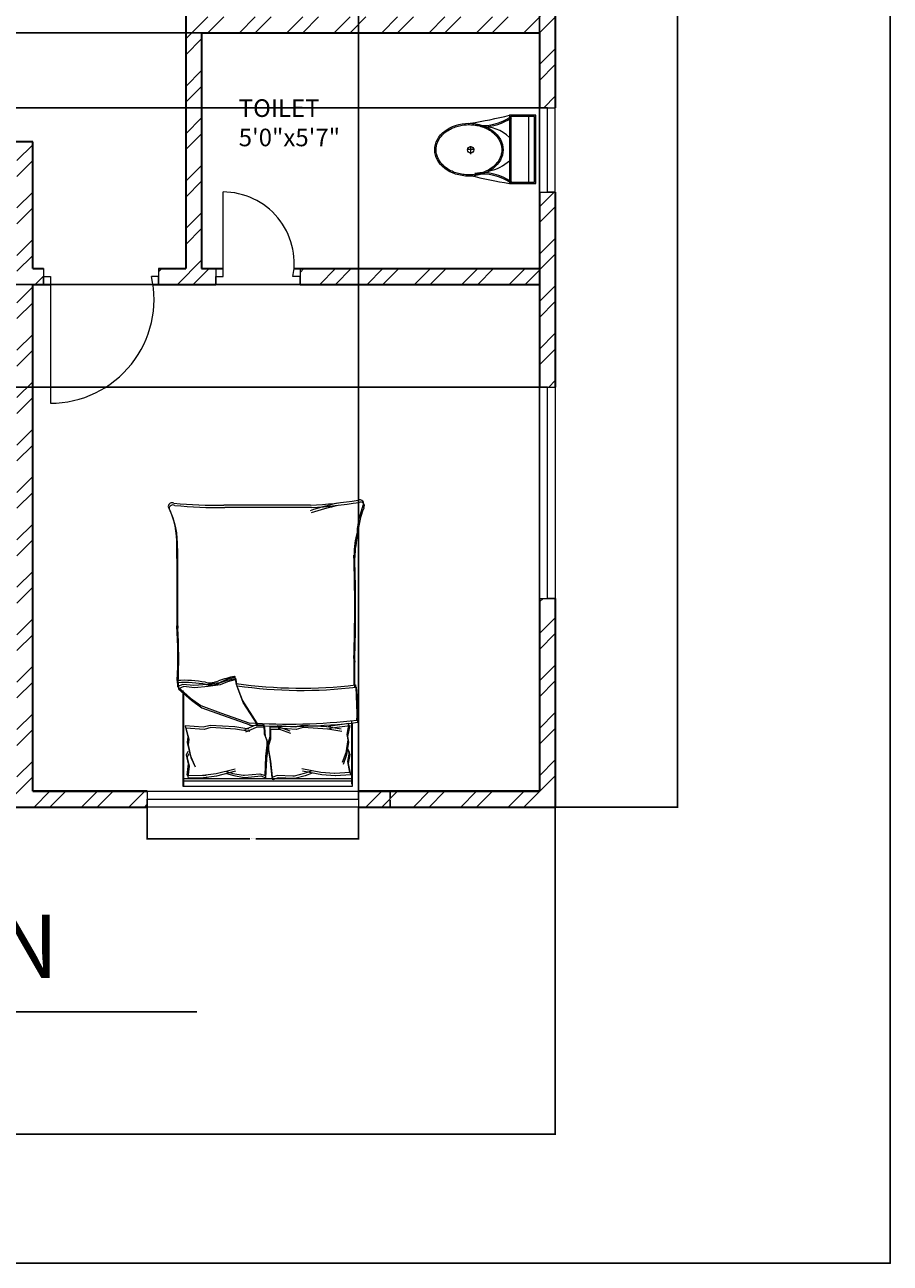
# Model space of a CAD drawing. Units: inches. Extents: x 1965 to 2673, y 1802 to 2669.
# Tile 5 of 16: x 2427 to 2673, y 1802 to 2154. Entities that reach past the tile are written whole.
import ezdxf

# ---------------------------------------------------------------- set-up
doc = ezdxf.new("R2010")
doc.units = ezdxf.units.IN
for name, color, linetype, lineweight in [('A-ANNO-DIMS', 2, 'Continuous', 18), ('A-ANNO-TTLB', 7, 'Continuous', 25), ('A-AREA-IDEN', 7, 'Continuous', 18), ('A-DOOR', 11, 'Continuous', 18), ('A-FLOR-FIXT', 9, 'Continuous', 18), ('A-FURN', 8, 'Continuous', 13), ('A-GLAZ', 181, 'Continuous', 18), ('A-WALL', 7, 'Continuous', 35), ('A-WALL-PATT', 252, 'Continuous', 13)]:
    doc.layers.add(name, color=color, linetype=linetype, lineweight=lineweight)
doc.styles.get("Standard").update_dxf_attribs({"font": 'arial.ttf'})
doc.dimstyles.get("Standard").update_dxf_attribs({"dimtxt": 0.18, "dimasz": 0.18, "dimexe": 0.18, "dimexo": 0.0625, "dimgap": 0.09, "dimtad": 0, "dimtih": 1, "dimtoh": 1, "dimdec": 4, "dimzin": 0, "dimdsep": 46, "dimtxsty": 'Standard', "dimcen": 0.09, "dimadec": 0, "dimazin": 0, "dimtfac": 1, "dimtdec": 4, "dimtofl": 0, "dimtmove": 0, "dimatfit": 3, "dimfxl": 1, "dimtolj": 1, "dimtzin": 0, "dimarcsym": 0})

# ---------------------------------------------------------------- blocks, each defined once
blk = doc.blocks.new('A$C31115884')
for p, q in [((283.1, 497.7), (223.4, 497.7)), ((257.5, 466.4), (257.5, 523.2)), ((0, 200), (0, 0)), ((520, 200), (0, 200)), ((10, 190), (10, 10)), ((510, 190), (10, 190)), ((510, 10), (510, 190)), ((520, 0), (520, 200)), ((510, 54.5), (0, 54.5)), ((10, 10), (510, 10)), ((0, 0), (520, 0))]:
    blk.add_line(p, q)
blk.add_circle((255.6, 496.4), 23.6)
for centre, radius, start, end in [((2777.7, -204.6), 2807, 165.4549, 171.71327), ((3237, 905), 2807, 188.28673, 194.5451), ((-294.5, 403.3), 364.7, 324.20913, 9.34987), ((-294.5, 403.3), 374.7, 324.20913, 9.34987), ((139.5, 406.2), 293.5, 315.84364, 2.65635), ((805.8, 403.3), 374.7, 179.20365, 215.79087), ((805.8, 403.3), 364.7, 170.65013, 215.79087), ((383.6, 406.2), 293.5, 190.27735, 224.15636)]:
    blk.add_arc(centre, radius, start, end)
blk.add_ellipse((256.2, 509.9), major_axis=(0, -260.7), ratio=0.772727)
blk.add_open_spline([(256.2, 259.2), (263.1, 259.2), (270, 259.7), (287.8, 262.3), (298.7, 265.1), (319.9, 273.1), (330.2, 278.4), (350.1, 291.1), (359.7, 298.7), (377.7, 315.9), (386.2, 325.5), (401.7, 346.6), (408.8, 358.1), (421.3, 382.5), (426.8, 395.5), (435.9, 422.4), (439.5, 436.4), (444.8, 465.1), (446.5, 479.7), (447.9, 509.2), (447.6, 524), (445, 553.3), (442.7, 567.8), (436.3, 596), (432.1, 609.7), (421.9, 636), (416, 648.6), (402.5, 672.1), (395, 683), (378.6, 703), (369.8, 712.1), (351.1, 728), (341.3, 734.8), (320.9, 746.2), (310.4, 750.7), (288.9, 757.3), (278, 759.4), (256, 761), (245, 760.6), (223.1, 757.2), (212.3, 754.3), (191.1, 746.1), (180.8, 740.7), (160.9, 727.8), (151.4, 720.1), (133.5, 702.7), (125.1, 693), (109.6, 671.7), (102.6, 660.2), (90.2, 635.7), (84.9, 622.7), (76, 595.6), (72.4, 581.6), (67.2, 552.9), (65.6, 538.2), (64.4, 508.8), (64.8, 494), (67.5, 464.7), (69.9, 450.2), (76.6, 422), (80.8, 408.3), (91.1, 382.2), (97.2, 369.7), (110.8, 346.3), (118.4, 335.4), (134.8, 315.6), (143.7, 306.7), (162.4, 290.9), (172.3, 284.2), (192.8, 273), (203.3, 268.6), (224.8, 262.2), (235.8, 260.2), (249.9, 259.3), (253, 259.2), (256.2, 259.2)], degree=3, knots=[0, 0, 0, 0, 0.110105, 0.110105, 0.285049, 0.285049, 0.459994, 0.459994, 0.634938, 0.634938, 0.809882, 0.809882, 0.984827, 0.984827, 1.159771, 1.159771, 1.334715, 1.334715, 1.50966, 1.50966, 1.684604, 1.684604, 1.859549, 1.859549, 2.034493, 2.034493, 2.209437, 2.209437, 2.384382, 2.384382, 2.559326, 2.559326, 2.73427, 2.73427, 2.909215, 2.909215, 3.084159, 3.084159, 3.259103, 3.259103, 3.434048, 3.434048, 3.608992, 3.608992, 3.783936, 3.783936, 3.958881, 3.958881, 4.133825, 4.133825, 4.30877, 4.30877, 4.483714, 4.483714, 4.658658, 4.658658, 4.833603, 4.833603, 5.008547, 5.008547, 5.183491, 5.183491, 5.358436, 5.358436, 5.53338, 5.53338, 5.708324, 5.708324, 5.883269, 5.883269, 6.058213, 6.058213, 6.233158, 6.233158, 6.283185, 6.283185, 6.283185, 6.283185])
blk = doc.blocks.new('BED-DOUBLE')
for p, q in [((3.47, 63.33), (3.47, 81.44)), ((3.47, 63.33), (3.47, 81.44)), ((3.47, 81.44), (51.49, 81.44)), ((51.26, 81.44), (51.26, 54.83)), ((51.26, 81.44), (51.26, 54.83)), ((51.49, 81.44), (51.49, 80.8)), ((3.47, 79.91), (51.26, 79.91)), ((3.47, 79.91), (51.26, 79.91)), ((3.7, 62.69), (3.7, 80.8)), ((3.7, 62.69), (3.7, 80.8)), ((3.7, 79.27), (51.49, 79.27)), ((3.7, 79.27), (51.49, 79.27)), ((3.89, 78.1), (8.17, 78.43)), ((3.89, 78.1), (8.17, 78.43)), ((3.89, 78.12), (4.47, 74.94)), ((3.89, 78.12), (4.47, 74.94)), ((4.12, 77.46), (8.4, 77.79)), ((4.12, 77.46), (8.4, 77.79)), ((4.12, 77.49), (4.7, 74.3)), ((4.12, 77.49), (4.7, 74.3)), ((8.17, 78.43), (8.28, 78.41)), ((8.17, 78.43), (8.28, 78.41)), ((8.28, 78.41), (12.1, 78.12)), ((8.28, 78.41), (12.1, 78.12)), ((8.4, 77.79), (8.51, 77.77)), ((8.4, 77.79), (8.51, 77.77)), ((8.51, 77.77), (12.33, 77.49)), ((8.51, 77.77), (12.33, 77.49)), ((12.1, 78.12), (17.6, 77.11)), ((12.1, 78.12), (17.6, 77.11)), ((12.33, 77.49), (17.82, 76.47)), ((12.33, 77.49), (17.82, 76.47)), ((14.85, 77.69), (16.87, 78.41)), ((14.85, 77.69), (16.87, 78.41)), ((15.08, 77.05), (17.1, 77.77)), ((15.08, 77.05), (17.1, 77.77)), ((16.87, 78.41), (19.76, 79.14)), ((16.87, 78.41), (19.76, 79.14)), ((17.1, 77.77), (19.99, 78.5)), ((17.1, 77.77), (19.99, 78.5)), ((19.76, 79.14), (20.09, 79.14)), ((19.76, 79.14), (20.09, 79.14)), ((19.99, 78.5), (20.31, 78.5)), ((19.99, 78.5), (20.31, 78.5)), ((20.09, 79.14), (24.53, 78.99)), ((20.09, 79.14), (24.53, 78.99)), ((20.31, 78.5), (24.76, 78.35)), ((20.31, 78.5), (24.76, 78.35)), ((24.53, 78.99), (25.98, 79.57)), ((24.53, 78.99), (25.98, 79.57)), ((24.76, 78.35), (26.21, 78.93)), ((24.76, 78.35), (26.21, 78.93)), ((25.98, 79.57), (26.56, 74.22)), ((25.98, 79.57), (26.56, 74.22)), ((26.21, 78.93), (26.78, 73.58)), ((26.21, 78.93), (26.78, 73.58)), ((27.97, 78.95), (27.73, 73.57)), ((27.97, 78.95), (27.73, 73.57)), ((28.2, 78.31), (27.96, 72.93)), ((28.2, 78.31), (27.96, 72.93)), ((29.45, 78.46), (27.97, 78.95)), ((29.45, 78.46), (27.97, 78.95)), ((29.68, 77.82), (28.2, 78.31)), ((29.68, 77.82), (28.2, 78.31)), ((33.88, 78.88), (29.45, 78.46)), ((33.88, 78.88), (29.45, 78.46)), ((34.11, 78.24), (29.68, 77.82)), ((34.11, 78.24), (29.68, 77.82)), ((34.2, 78.9), (33.88, 78.88)), ((34.2, 78.9), (33.88, 78.88)), ((34.43, 78.26), (34.11, 78.24)), ((34.43, 78.26), (34.11, 78.24)), ((37.13, 78.36), (34.2, 78.9)), ((37.13, 78.36), (34.2, 78.9)), ((37.36, 77.72), (34.43, 78.26)), ((37.36, 77.72), (34.43, 78.26)), ((41.91, 78.37), (36.49, 77.02)), ((41.91, 78.37), (36.49, 77.02)), ((42.14, 77.73), (36.72, 76.38)), ((42.14, 77.73), (36.72, 76.38)), ((39.2, 77.77), (37.13, 78.36)), ((39.19, 77.77), (37.13, 78.36)), ((39.42, 77.13), (37.36, 77.72)), ((39.42, 77.13), (37.36, 77.72)), ((45.71, 78.9), (41.91, 78.37)), ((45.71, 78.9), (41.91, 78.37)), ((45.94, 78.26), (42.14, 77.73)), ((45.94, 78.26), (42.14, 77.73)), ((50.11, 78.88), (44.7, 78.98)), ((44.7, 78.98), (45.71, 78.9)), ((50.11, 78.88), (44.7, 78.98)), ((44.7, 78.98), (45.71, 78.9)), ((50.34, 78.24), (44.93, 78.34)), ((44.93, 78.34), (45.94, 78.26)), ((50.34, 78.24), (44.93, 78.34)), ((44.93, 78.34), (45.94, 78.26)), ((50.11, 78.88), (49.73, 75.67)), ((50.11, 78.88), (49.73, 75.67)), ((50.34, 78.24), (49.96, 75.03)), ((50.34, 78.24), (49.96, 75.03)), ((51.49, 80.8), (51.49, 54.19)), ((51.49, 80.8), (51.49, 54.19)), ((4.47, 74.94), (4.03, 72.34)), ((4.47, 74.94), (4.03, 72.34)), ((4.7, 74.3), (4.26, 71.7)), ((4.7, 74.3), (4.26, 71.7)), ((5.05, 72.49), (6.06, 75.23)), ((5.05, 72.49), (6.06, 75.23)), ((5.27, 71.85), (6.29, 74.59)), ((5.27, 71.85), (6.29, 74.59)), ((26.56, 74.22), (27.13, 71.04)), ((26.56, 74.22), (27.13, 71.04)), ((49.3, 73.18), (48.12, 75.86)), ((49.3, 73.18), (48.12, 75.86)), ((49.53, 72.54), (48.35, 75.22)), ((49.53, 72.54), (48.35, 75.22)), ((49.73, 75.67), (50.32, 73.1)), ((49.73, 75.67), (50.32, 73.1)), ((49.96, 75.03), (50.55, 72.46)), ((49.96, 75.03), (50.55, 72.46)), ((4.03, 72.34), (4.61, 71.33)), ((4.03, 72.34), (4.61, 71.33)), ((4.26, 71.7), (4.84, 70.69)), ((4.26, 71.7), (4.84, 70.69)), ((4.47, 68.87), (5.05, 72.49)), ((4.47, 68.87), (5.05, 72.49)), ((4.7, 68.23), (5.27, 71.85)), ((4.7, 68.23), (5.27, 71.85)), ((26.78, 73.58), (27.36, 70.4)), ((26.78, 73.58), (27.36, 70.4)), ((27.13, 71.04), (27.13, 69.74)), ((27.13, 71.04), (27.13, 69.74)), ((27.73, 73.57), (27.35, 70.36)), ((27.73, 73.57), (27.35, 70.36)), ((27.36, 70.4), (27.36, 69.1)), ((27.36, 70.4), (27.36, 69.1)), ((27.96, 72.93), (27.58, 69.72)), ((27.96, 72.93), (27.58, 69.72)), ((50.11, 69.61), (49.3, 73.18)), ((50.11, 69.61), (49.3, 73.18)), ((50.34, 68.97), (49.53, 72.54)), ((50.34, 68.97), (49.53, 72.54)), ((50.32, 73.1), (49.81, 72.06)), ((50.32, 73.1), (49.81, 72.06)), ((50.55, 72.46), (50.04, 71.42)), ((50.55, 72.46), (50.04, 71.42)), ((4.18, 64.1), (4.76, 67.28)), ((4.18, 64.1), (4.76, 67.28)), ((4.76, 67.28), (4.47, 68.87)), ((4.76, 67.28), (4.47, 68.87)), ((4.99, 66.64), (4.7, 68.23)), ((4.99, 66.64), (4.7, 68.23)), ((27.13, 69.74), (26.56, 67.86)), ((27.13, 69.74), (26.56, 67.86)), ((26.56, 67.86), (26.56, 65.18)), ((26.56, 67.86), (26.56, 65.18)), ((27.36, 69.1), (26.78, 67.22)), ((27.36, 69.1), (26.78, 67.22)), ((26.78, 67.22), (26.78, 64.54)), ((26.78, 67.22), (26.78, 64.54)), ((27.35, 70.36), (27.43, 69.06)), ((27.35, 70.36), (27.43, 69.06)), ((27.43, 69.06), (28.13, 67.22)), ((27.43, 69.06), (28.13, 67.22)), ((27.58, 69.72), (27.66, 68.42)), ((27.58, 69.72), (27.66, 68.42)), ((27.66, 68.42), (28.35, 66.58)), ((27.66, 68.42), (28.35, 66.58)), ((28.13, 67.22), (28.29, 64.55)), ((28.13, 67.22), (28.29, 64.55)), ((49.92, 68.01), (50.11, 69.61)), ((49.92, 68.01), (50.11, 69.61)), ((50.69, 64.87), (49.92, 68.01)), ((50.69, 64.87), (49.92, 68.01)), ((50.15, 67.37), (50.34, 68.97)), ((50.15, 67.37), (50.34, 68.97)), ((50.92, 64.23), (50.15, 67.37)), ((50.92, 64.23), (50.15, 67.37)), ((9.28, 64.82), (4.18, 64.1)), ((9.28, 64.82), (4.18, 64.1)), ((4.41, 63.46), (4.99, 66.64)), ((4.41, 63.46), (4.99, 66.64)), ((9.5, 64.18), (4.41, 63.46)), ((9.5, 64.18), (4.41, 63.46)), ((6.38, 65.81), (10.41, 65.15)), ((6.38, 65.81), (10.41, 65.15)), ((6.6, 65.17), (10.64, 64.51)), ((6.61, 65.17), (10.64, 64.51)), ((10.41, 65.15), (9.28, 64.82)), ((10.41, 65.15), (9.28, 64.82)), ((10.64, 64.51), (9.5, 64.18)), ((10.64, 64.51), (9.5, 64.18)), ((10.41, 65.15), (17.42, 64.71)), ((10.41, 65.15), (17.42, 64.71)), ((10.64, 64.51), (17.65, 64.08)), ((10.64, 64.51), (17.65, 64.08)), ((17.42, 64.71), (19.38, 65.27)), ((17.42, 64.71), (19.38, 65.27)), ((17.65, 64.08), (19.61, 64.63)), ((17.65, 64.08), (19.61, 64.63)), ((19.38, 65.27), (24.51, 64.87)), ((19.38, 65.27), (24.51, 64.87)), ((19.61, 64.63), (24.74, 64.23)), ((19.61, 64.63), (24.74, 64.23)), ((24.1, 65.18), (20.95, 66.27)), ((24.1, 65.18), (20.95, 66.27)), ((24.33, 64.54), (21.18, 65.63)), ((24.33, 64.54), (21.18, 65.63)), ((26.56, 65.18), (24.1, 65.18)), ((26.56, 65.18), (24.1, 65.18)), ((26.78, 64.54), (24.33, 64.54)), ((26.78, 64.54), (24.33, 64.54)), ((28.29, 64.55), (30.75, 64.7)), ((28.29, 64.55), (30.75, 64.7)), ((28.35, 66.58), (28.52, 63.91)), ((28.35, 66.58), (28.52, 63.91)), ((28.52, 63.91), (30.97, 64.06)), ((28.52, 63.91), (30.97, 64.06)), ((30.25, 64.06), (34.44, 57.56)), ((30.25, 64.06), (34.44, 57.56)), ((30.48, 63.42), (34.67, 56.92)), ((30.48, 63.42), (34.67, 56.92)), ((30.75, 64.7), (33.82, 65.99)), ((30.75, 64.7), (33.82, 65.99)), ((30.97, 64.06), (34.04, 65.35)), ((30.97, 64.06), (34.04, 65.35)), ((40.64, 61.12), (32.3, 64.06)), ((40.64, 61.12), (32.3, 64.06)), ((40.87, 60.48), (32.53, 63.42)), ((40.87, 60.48), (32.53, 63.42)), ((32.56, 65.81), (36.59, 65.15)), ((32.56, 65.81), (36.59, 65.15)), ((32.79, 65.17), (36.82, 64.51)), ((32.79, 65.17), (36.82, 64.51)), ((36.59, 65.15), (43.6, 64.71)), ((36.59, 65.15), (43.6, 64.71)), ((36.82, 64.51), (43.83, 64.08)), ((36.82, 64.51), (43.83, 64.08)), ((43.6, 64.71), (45.56, 65.27)), ((43.6, 64.71), (45.56, 65.27)), ((43.83, 64.08), (45.79, 64.63)), ((43.83, 64.08), (45.79, 64.63)), ((45.56, 65.27), (50.69, 64.87)), ((45.56, 65.27), (50.69, 64.87)), ((45.79, 64.63), (50.92, 64.23)), ((45.79, 64.63), (50.92, 64.23)), ((46.21, 59.11), (40.64, 61.12)), ((46.21, 59.11), (40.64, 61.12)), ((46.44, 58.47), (40.87, 60.48)), ((46.44, 58.47), (40.87, 60.48)), ((34.44, 57.56), (36.15, 53.08)), ((34.44, 57.56), (36.15, 53.08)), ((34.67, 56.92), (36.38, 52.44)), ((34.67, 56.92), (36.38, 52.44)), ((49.16, 56.95), (46.21, 59.11)), ((49.16, 56.95), (46.21, 59.11)), ((49.39, 56.31), (46.44, 58.47)), ((49.39, 56.31), (46.44, 58.47)), ((52.86, 53.69), (49.16, 56.95)), ((52.86, 53.69), (49.16, 56.95)), ((53.09, 53.06), (49.39, 56.31)), ((53.09, 53.06), (49.39, 56.31)), ((36.15, 53.08), (36.46, 51.06)), ((36.15, 53.08), (36.46, 51.06)), ((40.95, 52.61), (44.36, 53.08)), ((40.95, 52.61), (44.36, 53.08)), ((44.36, 53.08), (48.23, 53.39)), ((44.36, 53.08), (48.23, 53.39)), ((48.23, 53.39), (51.33, 53.08)), ((48.23, 53.39), (51.33, 53.08)), ((51.33, 53.08), (52.86, 53.69)), ((51.33, 53.08), (52.86, 53.69)), ((51.55, 52.44), (53.09, 53.06)), ((51.55, 52.44), (53.09, 53.06)), ((52.94, 51.95), (52.86, 53.69, 3.87)), ((52.94, 51.95), (52.86, 53.69, 3.87)), ((53.17, 51.31), (53.09, 53.06, 3.87)), ((53.17, 51.31), (53.09, 53.06, 3.87)), ((36.38, 52.44), (36.69, 50.42)), ((36.38, 52.44), (36.69, 50.42)), ((36.46, 51.06), (38.94, 51.68)), ((36.46, 51.06), (38.94, 51.68)), ((36.69, 50.42), (39.16, 51.04)), ((36.69, 50.42), (39.16, 51.04)), ((38.94, 51.68), (40.95, 52.61)), ((38.94, 51.68), (40.95, 52.61)), ((39.16, 51.04), (41.18, 51.97)), ((39.16, 51.04), (41.18, 51.97)), ((41.18, 51.97), (44.58, 52.44)), ((41.18, 51.97), (44.58, 52.44)), ((44.58, 52.44), (48.46, 52.75)), ((44.58, 52.44), (48.46, 52.75)), ((48.46, 52.75), (51.55, 52.44)), ((48.46, 52.75), (51.55, 52.44)), ((15.06, 2.2), (39.67, 2.2)), ((15.06, 2.2), (39.67, 2.2)), ((15.29, 1.56), (39.9, 1.56)), ((15.29, 1.56), (39.9, 1.56))]:
    blk.add_line(p, q)
for centre, radius, start, end in [((21.35, -100.61), 164.97, 86.0865, 96.7821), ((21.35, -100.61), 164.97, 86.0865, 96.7821), ((21.58, -101.25), 164.97, 86.0865, 96.7821), ((21.58, -101.25), 164.97, 86.0865, 96.7821), ((85.16, 61.34), 83.31, 178.7218, 185.604), ((85.16, 61.34), 83.31, 178.7218, 185.604), ((85.39, 60.71), 83.31, 178.7218, 185.604), ((85.38, 60.71), 83.31, 178.7218, 185.604), ((17.75, -74.88), 129.02, 81.7845, 96.9006), ((17.75, -74.88), 129.02, 81.7845, 96.9006), ((17.98, -75.51), 129.02, 81.7845, 96.9006), ((17.98, -75.51), 129.02, 81.7845, 96.9006), ((-167.31, 50.27), 170.11, 358.4762, 1.0082), ((-167.31, 50.27), 170.11, 358.4762, 1.0082), ((-167.08, 49.63), 170.11, 358.4762, 1.0082), ((-167.08, 49.63), 170.11, 358.4762, 1.0082), ((36.63, 51), 0.185, 160.2464, 271.1377), ((36.63, 51), 0.185, 160.2464, 271.1377), ((31.15, 79.96), 29.65, 280.6617, 289.8806), ((31.15, 79.96), 29.65, 280.6617, 289.8806), ((36.86, 50.36), 0.185, 160.2464, 271.1377), ((36.86, 50.36), 0.185, 160.2464, 271.1377), ((31.38, 79.32), 29.65, 280.6617, 289.8806), ((31.38, 79.32), 29.65, 280.6617, 289.8806), ((43.74, 46.37), 6.22, 78.6608, 113.7384), ((43.74, 46.37), 6.22, 78.6608, 113.7384), ((43.97, 45.74), 6.22, 78.6608, 113.7384), ((43.97, 45.74), 6.22, 78.6608, 113.7384), ((51.32, 88.1), 36.18, 259.8763, 272.5657), ((51.32, 88.1), 36.18, 259.8763, 272.5657), ((51.55, 87.46), 36.18, 259.8763, 272.5657), ((51.55, 87.46), 36.18, 259.8763, 272.5657), ((182.26, 45.13), 129.5, 176.9791, 183.8365), ((182.26, 45.13), 129.5, 176.9791, 183.8365), ((182.49, 44.49), 129.5, 176.9791, 183.8365), ((182.49, 44.49), 129.5, 176.9791, 183.8365), ((484.82, 30.83), 482.31, 178.2277, 181.7185), ((484.82, 30.83), 482.31, 178.2277, 181.7185), ((485.05, 30.19), 482.31, 178.2277, 181.7185), ((485.05, 30.19), 482.31, 178.2277, 181.7185), ((-4508.75, 13.62), 4561.86, 0.00217, 0.28689), ((-4508.75, 13.62), 4561.86, 0.00217, 0.28689), ((-4508.52, 12.98), 4561.86, 0.00217, 0.28689), ((-4508.52, 12.98), 4561.86, 0.00217, 0.28689), ((-26.9, 16.93), 29.63, 346.0648, 358.9113), ((-26.9, 16.93), 29.63, 346.0648, 358.9113), ((-26.68, 16.29), 29.63, 346.0648, 358.9113), ((-26.68, 16.29), 29.63, 346.0648, 358.9113), ((76.15, 12.77), 23.07, 177.4714, 206.4681), ((76.15, 12.77), 23.07, 177.4714, 206.4681), ((76.38, 12.14), 23.07, 177.4714, 206.4681), ((76.38, 12.14), 23.07, 177.4714, 206.4681), ((-21.66, 11.17), 23.56, 337.9751, 356.652), ((-21.66, 11.17), 23.56, 337.9751, 356.652), ((-21.44, 10.53), 23.56, 337.9751, 356.652), ((-21.44, 10.53), 23.56, 337.9751, 356.652), ((-17.23, 105.15), 106.46, 283.3832, 287.7053), ((-17.23, 105.15), 106.46, 283.3832, 287.7053), ((1.08, 1.72), 1.09, 146.1736, 293.4781), ((1.08, 1.72), 1.09, 146.1736, 293.4781), ((1.31, 1.08), 1.09, 146.1736, 293.4781), ((1.31, 1.08), 1.09, 146.1736, 293.4781), ((21.42, -119.4), 121.76, 92.9958, 99.4091), ((21.42, -119.4), 121.76, 92.9958, 99.4091), ((21.65, -120.04), 121.76, 92.9958, 99.4091), ((21.65, -120.04), 121.76, 92.9958, 99.4091), ((-17, 104.51), 106.46, 283.3832, 287.7053), ((-17, 104.51), 106.46, 283.3832, 287.7053), ((41.15, -130.84), 133.04, 84.4998, 90.6351), ((41.15, -130.84), 133.04, 84.4998, 90.6351), ((41.38, -131.48), 133.04, 84.4998, 90.6351), ((41.37, -131.48), 133.04, 84.4998, 90.6351), ((54.4, 2.57), 1.1, 242.6588, 356.02), ((54.4, 2.57), 1.1, 242.6588, 356.02), ((54.63, 1.93), 1.1, 242.6588, 356.02), ((54.63, 1.93), 1.1, 242.6588, 356.02)]:
    blk.add_arc(centre, radius, start, end)
blk = doc.blocks.new('WIN-60IN')
for p, q in [((0, 4.5), (0, 0)), ((0, 4.5), (60, 4.5)), ((60, 2.25), (60, 4.5)), ((60, 4.5), (60, 0)), ((0, 0), (0, 2.25)), ((0, 2.25), (60, 2.25)), ((60, 0), (0, 0))]:
    blk.add_line(p, q)
blk = doc.blocks.new('WIN-24IN')
for p, q in [((0, 24), (4.5, 24)), ((0, 24), (0, 0)), ((4.5, 24), (2.25, 24)), ((2.25, 24), (2.25, 0)), ((4.5, 24), (4.5, 0)), ((2.25, 0), (0, 0)), ((0, 0), (4.5, 0))]:
    blk.add_line(p, q)
blk = doc.blocks.new('*D9')
at = {"layer": 'A-ANNO-DIMS', "color": 0, "lineweight": -2, "transparency": 16777216}
for p, q in [((2462.13, 1931.53), (2462.13, 1922.41)), ((2522.13, 1931.53), (2522.13, 1922.41)), ((2462.31, 1922.59), (2491.29, 1922.59)), ((2521.95, 1922.59), (2492.98, 1922.59))]:
    blk.add_line(p, q, dxfattribs=at)
at = {"layer": 'A-ANNO-DIMS', "color": 0, "transparency": 16777216}
for points in [[(2462.31, 1922.62), (2462.31, 1922.56), (2462.13, 1922.59)], [(2521.95, 1922.62), (2521.95, 1922.56), (2522.13, 1922.59)]]:
    blk.add_solid(points, dxfattribs=at)
at = {"layer": 'Defpoints', "color": 0, "transparency": 16777216}
for p in [(2462.13, 1931.59), (2522.13, 1931.59), (2522.13, 1922.59)]:
    blk.add_point(p, dxfattribs=at)
at = {"layer": 'A-ANNO-DIMS', "color": 0, "transparency": 16777216, "insert": (2492.13, 1922.59), "char_height": 0.18, "attachment_point": 5}
blk.add_mtext('\\A1;WIN. 60 TYP.', dxfattribs=at)
blk = doc.blocks.new('*D10')
at = {"layer": 'A-ANNO-DIMS', "color": 0, "lineweight": -2, "transparency": 16777216}
for p, q in [((2522.19, 1936.09), (2531.31, 1936.09)), ((2531.13, 1935.91), (2531.13, 1934.02)), ((2522.19, 1931.59), (2531.31, 1931.59)), ((2531.13, 1931.77), (2531.13, 1933.66))]:
    blk.add_line(p, q, dxfattribs=at)
at = {"layer": 'A-ANNO-DIMS', "color": 0, "transparency": 16777216}
for points in [[(2531.1, 1935.91), (2531.16, 1935.91), (2531.13, 1936.09)], [(2531.1, 1931.77), (2531.16, 1931.77), (2531.13, 1931.59)]]:
    blk.add_solid(points, dxfattribs=at)
at = {"layer": 'Defpoints', "color": 0, "transparency": 16777216}
for p in [(2522.13, 1936.09), (2531.13, 1936.09), (2522.13, 1931.59)]:
    blk.add_point(p, dxfattribs=at)
at = {"layer": 'A-ANNO-DIMS', "color": 0, "transparency": 16777216, "insert": (2531.13, 1933.84), "char_height": 0.18, "attachment_point": 5}
blk.add_mtext('\\A1;5 TYP.', dxfattribs=at)
blk = doc.blocks.new('*D25')
at = {"layer": 'A-ANNO-DIMS', "color": 0, "lineweight": -2, "transparency": 16777216}
for p, q in [((2047.09, 1931.53), (2047.09, 1838.49)), ((2578.09, 1931.53), (2578.09, 1838.49)), ((2047.27, 1838.67), (2312.32, 1838.67)), ((2577.91, 1838.67), (2312.86, 1838.67))]:
    blk.add_line(p, q, dxfattribs=at)
at = {"layer": 'A-ANNO-DIMS', "color": 0, "transparency": 16777216}
for points in [[(2047.27, 1838.7), (2047.27, 1838.64), (2047.09, 1838.67)], [(2577.91, 1838.7), (2577.91, 1838.64), (2578.09, 1838.67)]]:
    blk.add_solid(points, dxfattribs=at)
at = {"layer": 'Defpoints', "color": 0, "transparency": 16777216}
for p in [(2047.09, 1931.59), (2578.09, 1931.59), (2578.09, 1838.67)]:
    blk.add_point(p, dxfattribs=at)
at = {"layer": 'A-ANNO-DIMS', "color": 0, "transparency": 16777216, "insert": (2312.59, 1838.67), "char_height": 0.18, "attachment_point": 5}
blk.add_mtext('\\A1;531', dxfattribs=at)
blk = doc.blocks.new('*D26')
at = {"layer": 'A-ANNO-DIMS', "color": 0, "lineweight": -2, "transparency": 16777216}
for p, q in [((2578.16, 2565.59), (2613, 2565.59)), ((2612.82, 2565.41), (2612.82, 2248.77)), ((2612.82, 1931.77), (2612.82, 2248.41)), ((2578.16, 1931.59), (2613, 1931.59))]:
    blk.add_line(p, q, dxfattribs=at)
at = {"layer": 'A-ANNO-DIMS', "color": 0, "transparency": 16777216}
for points in [[(2612.79, 2565.41), (2612.85, 2565.41), (2612.82, 2565.59)], [(2612.79, 1931.77), (2612.85, 1931.77), (2612.82, 1931.59)]]:
    blk.add_solid(points, dxfattribs=at)
at = {"layer": 'Defpoints', "color": 0, "transparency": 16777216}
for p in [(2578.09, 2565.59), (2612.82, 2565.59), (2578.09, 1931.59)]:
    blk.add_point(p, dxfattribs=at)
at = {"layer": 'A-ANNO-DIMS', "color": 0, "transparency": 16777216, "insert": (2612.82, 2248.59), "char_height": 0.18, "attachment_point": 5}
blk.add_mtext('\\A1;634', dxfattribs=at)
blk = doc.blocks.new('*D44')
at = {"layer": 'A-ANNO-DIMS', "color": 0, "lineweight": -2, "transparency": 16777216}
for p, q in [((2522.13, 1936.15), (2522.13, 2600.5)), ((2522.31, 2600.32), (2547.47, 2600.32)), ((2573.41, 2600.32), (2548.26, 2600.32)), ((2573.59, 1936.15), (2573.59, 2600.5))]:
    blk.add_line(p, q, dxfattribs=at)
at = {"layer": 'A-ANNO-DIMS', "color": 0, "transparency": 16777216}
for points in [[(2522.31, 2600.35), (2522.31, 2600.29), (2522.13, 2600.32)], [(2573.41, 2600.35), (2573.41, 2600.29), (2573.59, 2600.32)]]:
    blk.add_solid(points, dxfattribs=at)
at = {"layer": 'Defpoints', "color": 0, "transparency": 16777216}
for p in [(2573.59, 2600.32), (2522.13, 1936.09), (2573.59, 1936.09)]:
    blk.add_point(p, dxfattribs=at)
at = {"layer": 'A-ANNO-DIMS', "color": 0, "transparency": 16777216, "insert": (2547.86, 2600.32), "char_height": 0.18, "attachment_point": 5}
blk.add_mtext('\\A1;51.46', dxfattribs=at)
blk = doc.blocks.new('*D45')
at = {"layer": 'A-ANNO-DIMS', "color": 0, "lineweight": -2, "transparency": 16777216}
for p, q in [((2573.53, 2080.09), (2012.19, 2080.09)), ((2012.37, 2079.91), (2012.37, 2065.68)), ((2012.37, 2051.08), (2012.37, 2065.31)), ((2573.53, 2050.9), (2012.19, 2050.9))]:
    blk.add_line(p, q, dxfattribs=at)
at = {"layer": 'A-ANNO-DIMS', "color": 0, "transparency": 16777216}
for points in [[(2012.34, 2079.91), (2012.4, 2079.91), (2012.37, 2080.09)], [(2012.34, 2051.08), (2012.4, 2051.08), (2012.37, 2050.9)]]:
    blk.add_solid(points, dxfattribs=at)
at = {"layer": 'Defpoints', "color": 0, "transparency": 16777216}
for p in [(2012.37, 2080.09), (2573.59, 2080.09), (2573.59, 2050.9)]:
    blk.add_point(p, dxfattribs=at)
at = {"layer": 'A-ANNO-DIMS', "color": 0, "transparency": 16777216, "insert": (2012.37, 2065.49), "char_height": 0.18, "attachment_point": 5}
blk.add_mtext('\\A1;29.19', dxfattribs=at)
blk = doc.blocks.new('*D46')
at = {"layer": 'A-ANNO-DIMS', "color": 0, "lineweight": -2, "transparency": 16777216}
for p, q in [((2573.53, 2151.59), (2012.19, 2151.59)), ((2012.37, 2151.41), (2012.37, 2141.12)), ((2012.37, 2130.47), (2012.37, 2140.76)), ((2573.53, 2130.29), (2012.19, 2130.29))]:
    blk.add_line(p, q, dxfattribs=at)
at = {"layer": 'A-ANNO-DIMS', "color": 0, "transparency": 16777216}
for points in [[(2012.34, 2151.41), (2012.4, 2151.41), (2012.37, 2151.59)], [(2012.34, 2130.47), (2012.4, 2130.47), (2012.37, 2130.29)]]:
    blk.add_solid(points, dxfattribs=at)
at = {"layer": 'Defpoints', "color": 0, "transparency": 16777216}
for p in [(2012.37, 2151.59), (2573.59, 2151.59), (2573.59, 2130.29)]:
    blk.add_point(p, dxfattribs=at)
at = {"layer": 'A-ANNO-DIMS', "color": 0, "transparency": 16777216, "insert": (2012.37, 2140.94), "char_height": 0.18, "attachment_point": 5}
blk.add_mtext('\\A1;21.3', dxfattribs=at)

msp = doc.modelspace()

# ---------------------------------------------------------------- hatches: boundary and pattern name
at = {"layer": 'A-WALL-PATT'}
h = msp.add_hatch(dxfattribs=at)
h.set_pattern_fill('ANSI32', color=256)
h.paths.add_polyline_path([(2051.5927, 2561.0914), (2076.7559, 2561.0914), (2076.7559, 2563.3414), (2076.7559, 2565.5914), (2047.0927, 2565.5914), (2047.0927, 2518.3824), (2051.5927, 2518.3824)])
h.paths.add_polyline_path([(2051.5927, 2458.3824), (2049.3427, 2458.3824), (2047.0927, 2458.3824), (2047.0927, 2412.5914), (2248.0927, 2412.5914), (2248.0927, 2268.5914), (2252.5927, 2268.5914), (2252.5927, 2412.5914), (2252.5927, 2421.0404), (2250.3427, 2421.0404), (2248.0927, 2421.0404), (2248.0927, 2417.0914), (2051.5927, 2417.0914)])
h.paths.add_polyline_path([(2211.4933, 2268.5914), (2104.0927, 2268.5914), (2104.0927, 2272.4654), (2101.8427, 2272.4654), (2099.5927, 2272.4654), (2099.5927, 2268.5914), (2051.5927, 2268.5914), (2051.5927, 2264.0914), (2147.5927, 2264.0914), (2147.5927, 2259.8893), (2152.0927, 2259.8893), (2152.0927, 2264.0914), (2211.4933, 2264.0914), (2211.4933, 2266.3414)])
h.paths.add_polyline_path([(2104.0927, 2376.0914), (2099.5927, 2376.0914), (2047.0927, 2376.0914), (2047.0927, 2333.0682), (2051.5927, 2333.0682), (2051.5927, 2371.5914), (2099.5927, 2371.5914), (2099.5927, 2293.6123), (2104.0927, 2293.6123)], flags=17)
h.paths.add_polyline_path([(2051.5927, 2309.0682), (2047.0927, 2309.0682), (2047.0927, 2233.5821), (2051.5927, 2233.5821)])
h.paths.add_polyline_path([(2104.0927, 2412.5914), (2099.5927, 2412.5914), (2099.5927, 2376.0914), (2104.0927, 2376.0914)], flags=17)
h.paths.add_polyline_path([(2290.1254, 2268.5914), (2242.4924, 2268.5914), (2242.4924, 2264.0914), (2290.1254, 2264.0914), (2290.1254, 2266.3414)])
h.paths.add_polyline_path([(2284.653, 2264.0914), (2280.153, 2264.0914), (2280.153, 2161.6826), (2284.653, 2161.6826)])
h.paths.add_polyline_path([(2578.0927, 2329.4656), (2573.5927, 2329.4656), (2573.5927, 2268.5914), (2525.5927, 2268.5914), (2525.5927, 2271.9222), (2523.3427, 2271.9222), (2521.0927, 2271.9222), (2521.0927, 2268.5914), (2324.2835, 2268.5914), (2324.2835, 2264.0914), (2329.0927, 2264.0914), (2329.0927, 2259.4977), (2333.5927, 2259.4977), (2333.5927, 2264.0914), (2473.0927, 2264.0914), (2473.0927, 2259.9371), (2477.5927, 2259.9371), (2477.5927, 2264.0914), (2573.5927, 2264.0914), (2573.5927, 2235.5751), (2578.0927, 2235.5751)])
h.paths.add_polyline_path([(2377.0927, 2412.5914), (2578.0927, 2412.5914), (2578.0927, 2444.2286), (2575.8427, 2444.2286), (2573.5927, 2444.2286), (2573.5927, 2417.0914), (2429.5927, 2417.0914), (2377.0927, 2417.0914), (2377.0927, 2421.7443), (2372.5927, 2421.7443), (2372.5927, 2268.5914), (2377.0927, 2268.5914)])
h.paths.add_polyline_path([(2525.5927, 2371.5914), (2573.5927, 2371.5914), (2573.5927, 2353.4656), (2578.0927, 2353.4656), (2578.0927, 2376.0914), (2525.5927, 2376.0914), (2521.0927, 2376.0914), (2521.0927, 2290.6472), (2525.5927, 2290.6472)], flags=17)
h.paths.add_polyline_path([(2477.5927, 2236.4106), (2475.3427, 2236.4106), (2473.0927, 2236.4106), (2473.0927, 2084.5914), (2465.3309, 2084.5914), (2465.3309, 2080.0914), (2481.6764, 2080.0914), (2481.6764, 2082.3414), (2481.6764, 2084.5914), (2477.5927, 2084.5914), (2477.5927, 2151.5914), (2573.5927, 2151.5914), (2573.5927, 2130.2907), (2578.0927, 2130.2907), (2578.0927, 2199.5751), (2575.8427, 2199.5751), (2573.5927, 2199.5751), (2573.5927, 2156.0914), (2477.5927, 2156.0914)])
h.paths.add_polyline_path([(2573.5927, 2084.5914), (2505.5513, 2084.5914), (2505.5513, 2080.0914), (2573.5927, 2080.0914)], flags=17)
h.paths.add_polyline_path([(2578.0927, 2106.2907), (2575.8427, 2106.2907), (2573.5927, 2106.2907), (2573.5927, 2050.8986), (2578.0927, 2050.8986)])
h.paths.add_polyline_path([(2578.0927, 1990.8986), (2575.8427, 1990.8986), (2573.5927, 1990.8986), (2573.5927, 1936.0914), (2522.132, 1936.0914), (2522.132, 1931.5914), (2578.0927, 1931.5914)])
h.paths.add_polyline_path([(2462.132, 1936.0914), (2429.5927, 1936.0914), (2429.5927, 2080.0914), (2432.623, 2080.0914), (2432.623, 2082.3414), (2432.623, 2084.5914), (2429.5927, 2084.5914), (2429.5927, 2120.5914), (2333.5927, 2120.5914), (2333.5927, 2229.3125), (2331.3427, 2229.3125), (2329.0927, 2229.3125), (2329.0927, 2116.0914), (2425.0927, 2116.0914), (2425.0927, 1936.0914), (2346.4058, 1936.0914), (2346.4058, 1931.5914), (2462.132, 1931.5914), (2462.132, 1933.8414)])
h.paths.add_polyline_path([(2211.767, 1933.8414), (2211.767, 1936.0914), (2200.0927, 1936.0914), (2200.0927, 2080.0914), (2200.0927, 2116.0914), (2284.653, 2116.0914), (2284.653, 2130.591), (2282.403, 2130.591), (2280.153, 2130.591), (2280.153, 2120.5914), (2200.0927, 2120.5914), (2195.5927, 2120.5914), (2195.5927, 2080.0914), (2195.5927, 1936.0914), (2139.0533, 1936.0914), (2139.0533, 1931.5914), (2211.767, 1931.5914)])
h.paths.add_polyline_path([(2282.2502, 1933.8414), (2282.2502, 1936.0914), (2259.767, 1936.0914), (2259.767, 1931.5914), (2282.2502, 1931.5914)], flags=17)
h.paths.add_polyline_path([(2051.5927, 1987.096), (2049.3427, 1987.096), (2047.0927, 1987.096), (2047.0927, 1931.5914), (2079.0533, 1931.5914), (2079.0533, 1933.8414), (2079.0533, 1936.0914), (2051.5927, 1936.0914)])
h.paths.add_polyline_path([(2051.5927, 2197.5821), (2049.3427, 2197.5821), (2047.0927, 2197.5821), (2047.0927, 2141.952), (2051.5927, 2141.952), (2051.5927, 2151.5914), (2147.5927, 2151.5914), (2147.5927, 2084.5914), (2144.3652, 2084.5914), (2144.3652, 2080.0914), (2155.9662, 2080.0914), (2155.9662, 2082.3414), (2155.9662, 2084.5914), (2152.0927, 2084.5914), (2152.0927, 2239.4921), (2149.8427, 2239.4921), (2147.5927, 2239.4921), (2147.5927, 2156.0914), (2051.5927, 2156.0914)])
h.paths.add_polyline_path([(2051.5927, 2080.0914), (2123.8575, 2080.0914), (2123.8575, 2082.3414), (2123.8575, 2084.5914), (2051.5927, 2084.5914), (2051.5927, 2117.952), (2047.0927, 2117.952), (2047.0927, 2047.096), (2051.5927, 2047.096)])
h = msp.add_hatch(dxfattribs=at)
h.set_pattern_fill('ANSI32', color=256)
h.paths.add_polyline_path([(2210.2316, 2563.3414), (2210.2316, 2565.5914), (2136.7559, 2565.5914), (2136.7559, 2561.0914), (2195.5927, 2561.0914), (2195.5927, 2485.8604), (2200.0927, 2485.8604), (2200.0927, 2561.0914), (2210.2316, 2561.0914)])
h.paths.add_polyline_path([(2285.9734, 2565.5914), (2234.2316, 2565.5914), (2234.2316, 2561.0914), (2248.0927, 2561.0914), (2248.0927, 2462.0914), (2200.0927, 2462.0914), (2200.0927, 2465.2357), (2197.8427, 2465.2357), (2195.5927, 2465.2357), (2195.5927, 2457.5914), (2248.0927, 2457.5914), (2248.0927, 2452.628), (2252.5927, 2452.628), (2252.5927, 2457.5914), (2257.5156, 2457.5914), (2257.5156, 2459.8414), (2257.5156, 2462.0914), (2252.5927, 2462.0914), (2252.5927, 2561.0914), (2285.9734, 2561.0914)])
h.paths.add_polyline_path([(2213.1374, 1872.8885), (2461.061, 1872.8885), (2461.061, 1909.9813), (2213.1374, 1909.9813)], flags=9)
h.paths.add_polyline_path([(2328.4056, 1942.3944), (2340.6089, 1942.3944), (2340.6089, 1952.6979), (2328.4056, 1952.6979)], flags=9)
h.paths.add_polyline_path([(2353.5759, 2030.9808), (2376.6455, 2030.9808), (2376.6455, 2041.2844), (2353.5759, 2041.2844)], flags=9)
h.paths.add_polyline_path([(2289.989, 2074.1041), (2326.916, 2074.1041), (2326.916, 2092.7615), (2289.989, 2092.7615)], flags=9)
h.paths.add_polyline_path([(2497.9, 2052.8638), (2548.3741, 2052.8638), (2548.3741, 2071.5212), (2497.9, 2071.5212)], flags=9)
h.paths.add_polyline_path([(2486.59, 2116.4883), (2515.7475, 2116.4883), (2515.7475, 2135.1456), (2486.59, 2135.1456)], flags=9)
h.paths.add_polyline_path([(2497.3007, 2181.2877), (2530.459, 2181.2877), (2530.459, 2199.945), (2497.3007, 2199.945)], flags=9)
h.paths.add_polyline_path([(2288.237, 2190.3228), (2324.1238, 2190.3228), (2324.1238, 2208.9802), (2288.237, 2208.9802)], flags=9)
h.paths.add_polyline_path([(2350.806, 2127.8307), (2387.733, 2127.8307), (2387.733, 2146.488), (2350.806, 2146.488)], flags=9)
h.paths.add_polyline_path([(2530.3237, 2315.2679), (2559.5563, 2315.2679), (2559.5563, 2333.9252), (2530.3237, 2333.9252)], flags=9)
h.paths.add_polyline_path([(2418.419, 2383.4707), (2468.2894, 2383.4707), (2468.2894, 2402.1281), (2418.419, 2402.1281)], flags=9)
h.paths.add_polyline_path([(2327.4503, 2399.0281), (2364.3773, 2399.0281), (2364.3773, 2417.6854), (2327.4503, 2417.6854)], flags=9)
h.paths.add_polyline_path([(2147.9722, 2271.4601), (2197.8426, 2271.4601), (2197.8426, 2290.1174), (2147.9722, 2290.1174)], flags=9)
h.paths.add_polyline_path([(2474.3875, 2421.594), (2524.8616, 2421.594), (2524.8616, 2440.2514), (2474.3875, 2440.2514)], flags=9)
h.paths.add_polyline_path([(2063.9863, 2052.9059), (2114.4604, 2052.9059), (2114.4604, 2071.5632), (2063.9863, 2071.5632)], flags=9)
h.paths.add_polyline_path([(2200.3335, 2133.7067), (2237.2605, 2133.7067), (2237.2605, 2152.364), (2200.3335, 2152.364)], flags=9)
h.paths.add_polyline_path([(2080.5973, 2184.636), (2113.8681, 2184.636), (2113.8681, 2203.2933), (2080.5973, 2203.2933)], flags=9)
h.paths.add_polyline_path([(2102.4918, 2116.4497), (2131.6494, 2116.4497), (2131.6494, 2135.107), (2102.4918, 2135.107)], flags=9)
h.paths.add_polyline_path([(2056.2753, 2308.5576), (2085.5079, 2308.5576), (2085.5079, 2327.2149), (2056.2753, 2327.2149)], flags=9)
h.paths.add_polyline_path([(2385.619, 2500.9729), (2414.8516, 2500.9729), (2414.8516, 2519.6303), (2385.619, 2519.6303)], flags=9)
h.paths.add_polyline_path([(2286.6643, 2508.6826), (2320.0715, 2508.6826), (2320.0715, 2527.34), (2286.6643, 2527.34)], flags=9)
h.paths.add_polyline_path([(2206.5604, 2500.7243), (2235.793, 2500.7243), (2235.793, 2519.3817), (2206.5604, 2519.3817)], flags=25)
h.paths.add_polyline_path([(2062.6644, 2424.4027), (2112.5348, 2424.4027), (2112.5348, 2443.0601), (2062.6644, 2443.0601)], flags=9)
h = msp.add_hatch(dxfattribs=at)
h.set_pattern_fill('ANSI32', color=256)
h.paths.add_polyline_path([(2429.5927, 2468.6101), (2427.3427, 2468.6101), (2425.0927, 2468.6101), (2425.0927, 2462.0914), (2377.0927, 2462.0914), (2377.0927, 2561.0914), (2390.4173, 2561.0914), (2390.4173, 2565.5914), (2321.9734, 2565.5914), (2321.9734, 2561.0914), (2372.5927, 2561.0914), (2372.5927, 2462.0914), (2281.6605, 2462.0914), (2281.6605, 2457.5914), (2372.5927, 2457.5914), (2372.5927, 2451.3316), (2377.0927, 2451.3316), (2377.0927, 2457.5914), (2429.5927, 2457.5914)])
h.paths.add_polyline_path([(2480.8929, 2565.5914), (2414.4173, 2565.5914), (2414.4173, 2561.0914), (2425.0927, 2561.0914), (2425.0927, 2489.9153), (2429.5927, 2489.9153), (2429.5927, 2561.0914), (2480.8929, 2561.0914), (2480.8929, 2563.3414)])
h.paths.add_polyline_path([(2213.1374, 1872.8885), (2461.061, 1872.8885), (2461.061, 1909.9813), (2213.1374, 1909.9813)], flags=9)
h.paths.add_polyline_path([(2328.4056, 1942.3944), (2340.6089, 1942.3944), (2340.6089, 1952.6979), (2328.4056, 1952.6979)], flags=9)
h.paths.add_polyline_path([(2353.5759, 2030.9808), (2376.6455, 2030.9808), (2376.6455, 2041.2844), (2353.5759, 2041.2844)], flags=9)
h.paths.add_polyline_path([(2289.989, 2074.1041), (2326.916, 2074.1041), (2326.916, 2092.7615), (2289.989, 2092.7615)], flags=9)
h.paths.add_polyline_path([(2497.9, 2052.8638), (2548.3741, 2052.8638), (2548.3741, 2071.5212), (2497.9, 2071.5212)], flags=9)
h.paths.add_polyline_path([(2486.59, 2116.4883), (2515.7475, 2116.4883), (2515.7475, 2135.1456), (2486.59, 2135.1456)], flags=9)
h.paths.add_polyline_path([(2497.3007, 2181.2877), (2530.459, 2181.2877), (2530.459, 2199.945), (2497.3007, 2199.945)], flags=9)
h.paths.add_polyline_path([(2288.237, 2190.3228), (2324.1238, 2190.3228), (2324.1238, 2208.9802), (2288.237, 2208.9802)], flags=9)
h.paths.add_polyline_path([(2350.806, 2127.8307), (2387.733, 2127.8307), (2387.733, 2146.488), (2350.806, 2146.488)], flags=9)
h.paths.add_polyline_path([(2530.3237, 2315.2679), (2559.5563, 2315.2679), (2559.5563, 2333.9252), (2530.3237, 2333.9252)], flags=9)
h.paths.add_polyline_path([(2418.419, 2383.4707), (2468.2894, 2383.4707), (2468.2894, 2402.1281), (2418.419, 2402.1281)], flags=9)
h.paths.add_polyline_path([(2327.4503, 2399.0281), (2364.3773, 2399.0281), (2364.3773, 2417.6854), (2327.4503, 2417.6854)], flags=9)
h.paths.add_polyline_path([(2147.9722, 2271.4601), (2197.8426, 2271.4601), (2197.8426, 2290.1174), (2147.9722, 2290.1174)], flags=9)
h.paths.add_polyline_path([(2474.3875, 2421.594), (2524.8616, 2421.594), (2524.8616, 2440.2514), (2474.3875, 2440.2514)], flags=9)
h.paths.add_polyline_path([(2063.9863, 2052.9059), (2114.4604, 2052.9059), (2114.4604, 2071.5632), (2063.9863, 2071.5632)], flags=9)
h.paths.add_polyline_path([(2200.3335, 2133.7067), (2237.2605, 2133.7067), (2237.2605, 2152.364), (2200.3335, 2152.364)], flags=9)
h.paths.add_polyline_path([(2080.5973, 2184.636), (2113.8681, 2184.636), (2113.8681, 2203.2933), (2080.5973, 2203.2933)], flags=9)
h.paths.add_polyline_path([(2102.4918, 2116.4497), (2131.6494, 2116.4497), (2131.6494, 2135.107), (2102.4918, 2135.107)], flags=9)
h.paths.add_polyline_path([(2056.2753, 2308.5576), (2085.5079, 2308.5576), (2085.5079, 2327.2149), (2056.2753, 2327.2149)], flags=9)
h.paths.add_polyline_path([(2385.619, 2500.9729), (2414.8516, 2500.9729), (2414.8516, 2519.6303), (2385.619, 2519.6303)], flags=25)
h.paths.add_polyline_path([(2286.6643, 2508.6826), (2320.0715, 2508.6826), (2320.0715, 2527.34), (2286.6643, 2527.34)], flags=25)
h.paths.add_polyline_path([(2206.5604, 2500.7243), (2235.793, 2500.7243), (2235.793, 2519.3817), (2206.5604, 2519.3817)], flags=9)
h.paths.add_polyline_path([(2062.6644, 2424.4027), (2112.5348, 2424.4027), (2112.5348, 2443.0601), (2062.6644, 2443.0601)], flags=9)

# ---------------------------------------------------------------- linework, layer by layer
at = {"layer": 'A-ANNO-TTLB'}
msp.add_line((2201.9386, 1873.3965), (2476.233, 1873.3965), dxfattribs=at)
msp.add_lwpolyline([(1964.5703, 2669.282), (2673.2605, 2669.282), (2673.2605, 1802.0221), (1964.5703, 1802.0221)], close=True, dxfattribs=at)
at = {"layer": 'A-DOOR'}
for p, q in [((2483.6764, 2082.3414), (2483.6764, 2106.3414)), ((2432.623, 2084.5914), (2432.623, 2080.0914)), ((2465.3309, 2084.5914), (2465.3309, 2080.0914)), ((2481.6764, 2084.5914), (2481.6764, 2080.0914)), ((2505.5513, 2084.5914), (2505.5513, 2080.0914)), ((2432.623, 2080.0914), (2432.623, 2082.3414)), ((2432.623, 2082.3414), (2434.623, 2082.3414)), ((2434.623, 2082.3414), (2434.623, 2046.3414)), ((2465.3309, 2082.3414), (2463.3309, 2082.3414)), ((2465.3309, 2080.0914), (2465.3309, 2082.3414)), ((2481.6764, 2080.0914), (2481.6764, 2082.3414)), ((2481.6764, 2082.3414), (2483.6764, 2082.3414)), ((2505.5513, 2082.3414), (2503.5513, 2082.3414)), ((2505.5513, 2080.0914), (2505.5513, 2082.3414))]:
    msp.add_line(p, q, dxfattribs=at)
for centre, radius, start, end in [((2483.6764, 2086.112), 20.2294, 349.257709, 90), ((2434.623, 2075.7878), 29.4464, 270, 12.85948)]:
    msp.add_arc(centre, radius, start, end, dxfattribs=at)
at = {"layer": 'A-WALL'}
for p, q in [((2473.0927, 2236.4106), (2473.0927, 2084.5914)), ((2578.0927, 2199.5751), (2578.0927, 2130.2907)), ((2477.5927, 2151.5914), (2573.5927, 2151.5914)), ((2477.5927, 2151.5914), (2477.5927, 2084.5914)), ((2573.5927, 2151.5914), (2573.5927, 2130.2907)), ((2429.5927, 2120.5914), (2333.5927, 2120.5914)), ((2429.5927, 2084.5914), (2429.5927, 2120.5914)), ((2573.5927, 2106.2907), (2573.5927, 2050.8986)), ((2578.0927, 2106.2907), (2578.0927, 2050.8986)), ((2429.5927, 2084.5914), (2432.623, 2084.5914)), ((2465.3309, 2084.5914), (2473.0927, 2084.5914)), ((2477.5927, 2084.5914), (2483.6764, 2084.5914)), ((2503.8486, 2084.5914), (2573.5927, 2084.5914)), ((2429.5927, 1936.0914), (2429.5927, 2080.0914)), ((2429.5927, 2080.0914), (2434.623, 2080.0914)), ((2463.7532, 2080.0914), (2481.6764, 2080.0914)), ((2505.5513, 2080.0914), (2573.5927, 2080.0914)), ((2573.5927, 1990.8986), (2573.5927, 1936.0914)), ((2578.0927, 1990.8986), (2578.0927, 1931.5914)), ((2429.5927, 1936.0914), (2462.132, 1936.0914)), ((2462.132, 1936.0914), (2429.5927, 1936.0914)), ((2573.5927, 1936.0914), (2522.132, 1936.0914)), ((2522.132, 1936.0914), (2573.5927, 1936.0914)), ((2346.4058, 1931.5914), (2462.132, 1931.5914)), ((2522.132, 1931.5914), (2578.0927, 1931.5914))]:
    msp.add_line(p, q, dxfattribs=at)

# ---------------------------------------------------------------- block references
at = {"layer": 'A-FLOR-FIXT', "xscale": 0.0372717239612423, "yscale": 0.0372717239612423, "zscale": 0.0372717239612423, "rotation": 89.99999999999999}
msp.add_blockref('A$C31115884', (2572.5539, 2108.7864), dxfattribs=at)
at = {"layer": 'A-FURN', "rotation": 180}
msp.add_blockref('BED-DOUBLE', (2523.8435, 2018.8951), dxfattribs=at)
at = {"layer": 'A-GLAZ', "extrusion": (0, 0, -1), "zscale": -1, "rotation": 180}
msp.add_blockref('WIN-24IN', (-2573.59, 2130.2863), dxfattribs=at)
at = {"layer": 'A-GLAZ', "rotation": 90}
msp.add_blockref('WIN-60IN', (2578.0941, 1990.9027), dxfattribs=at)
at = {"layer": 'A-GLAZ'}
msp.add_blockref('WIN-60IN', (2462.136, 1931.59), dxfattribs=at)

# ---------------------------------------------------------------- texts
at = {"layer": 'A-ANNO-TTLB', "insert": (2219.7001, 1901.0365), "char_height": 18, "attachment_point": 1}
msp.add_mtext_dynamic_manual_height_columns('FIRST FLOOR PLAN', width=462.606856, gutter_width=12.5, heights=[0], dxfattribs=at)
at = {"layer": 'A-AREA-IDEN', "insert": (2488.1299, 2132.661), "char_height": 5, "attachment_point": 1}
msp.add_mtext_dynamic_manual_height_columns('TOILET\\P5\'0"x5\'7"', width=240.55235, gutter_width=12.5, heights=[0], dxfattribs=at)

# ---------------------------------------------------------------- dimensions: what is measured, and where the dimension line sits
at = {"layer": 'A-ANNO-DIMS'}
for base, p1, p2, override, picture, middle in [((2573.5927, 2600.3164), (2522.132, 1936.0914), (2573.5927, 1936.0914), {"dimdec": 2, "dimlfac": 1, "dimrnd": 0, "dimzin": 0, "dimdsep": 46, "dimlunit": 2}, '*D44', (2547.8623, 2600.3164)), ((2578.0927, 1838.6715), (2047.0927, 1931.5914), (2578.0927, 1931.5914), {"dimdec": 0, "dimlfac": 1, "dimrnd": 0, "dimzin": 0, "dimdsep": 46, "dimlunit": 2}, '*D25', (2312.5927, 1838.6715))]:
    dim = msp.add_linear_dim(base=base, p1=p1, p2=p2, dimstyle='Standard', override=override, dxfattribs=at)
    dim.commit()
    dim.dimension.update_dxf_attribs({"geometry": picture, "text_midpoint": middle})
for base, p1, p2, override, picture, middle in [((2612.8177, 2565.5914), (2578.0927, 1931.5914), (2578.0927, 2565.5914), {"dimdec": 0, "dimlfac": 1, "dimrnd": 0, "dimzin": 0, "dimdsep": 46, "dimlunit": 2}, '*D26', (2612.8177, 2248.5914)), ((2012.3677, 2151.5914), (2573.5927, 2130.2907), (2573.5927, 2151.5914), {"dimdec": 1, "dimlfac": 1, "dimrnd": 0, "dimzin": 0, "dimdsep": 46, "dimlunit": 2}, '*D46', (2012.3677, 2140.941)), ((2012.3677, 2080.0914), (2573.5927, 2050.8986), (2573.5927, 2080.0914), {"dimdec": 2, "dimlfac": 1, "dimrnd": 0, "dimzin": 0, "dimdsep": 46, "dimlunit": 2}, '*D45', (2012.3677, 2065.495))]:
    dim = msp.add_linear_dim(base=base, p1=p1, p2=p2, angle=90, dimstyle='Standard', override=override, dxfattribs=at)
    dim.commit()
    dim.dimension.update_dxf_attribs({"geometry": picture, "text_midpoint": middle})
dim = msp.add_linear_dim(base=(2531.1319552685, 1936.0913673804), p1=(2522.1319552685, 1931.5913673804), p2=(2522.1319552685, 1936.0913673804), angle=90, text='<> TYP.', dimstyle='Standard', override={"dimdec": 0, "dimlfac": 1, "dimrnd": 0, "dimzin": 0, "dimdsep": 46, "dimlunit": 2}, dxfattribs=at)
dim.commit()
dim.dimension.update_dxf_attribs({"geometry": '*D10', "text_midpoint": (2531.1319552685, 1933.8413673804)})
dim = msp.add_linear_dim(base=(2522.132, 1922.5914), p1=(2462.132, 1931.5914), p2=(2522.132, 1931.5914), text='WIN. <> TYP.', dimstyle='Standard', override={"dimdec": 0, "dimlfac": 1, "dimrnd": 0, "dimzin": 0, "dimdsep": 46, "dimlunit": 2}, dxfattribs=at)
dim.commit()
dim.dimension.update_dxf_attribs({"geometry": '*D9', "text_midpoint": (2492.132, 1922.5914)})

doc.saveas('drawing.dxf')
